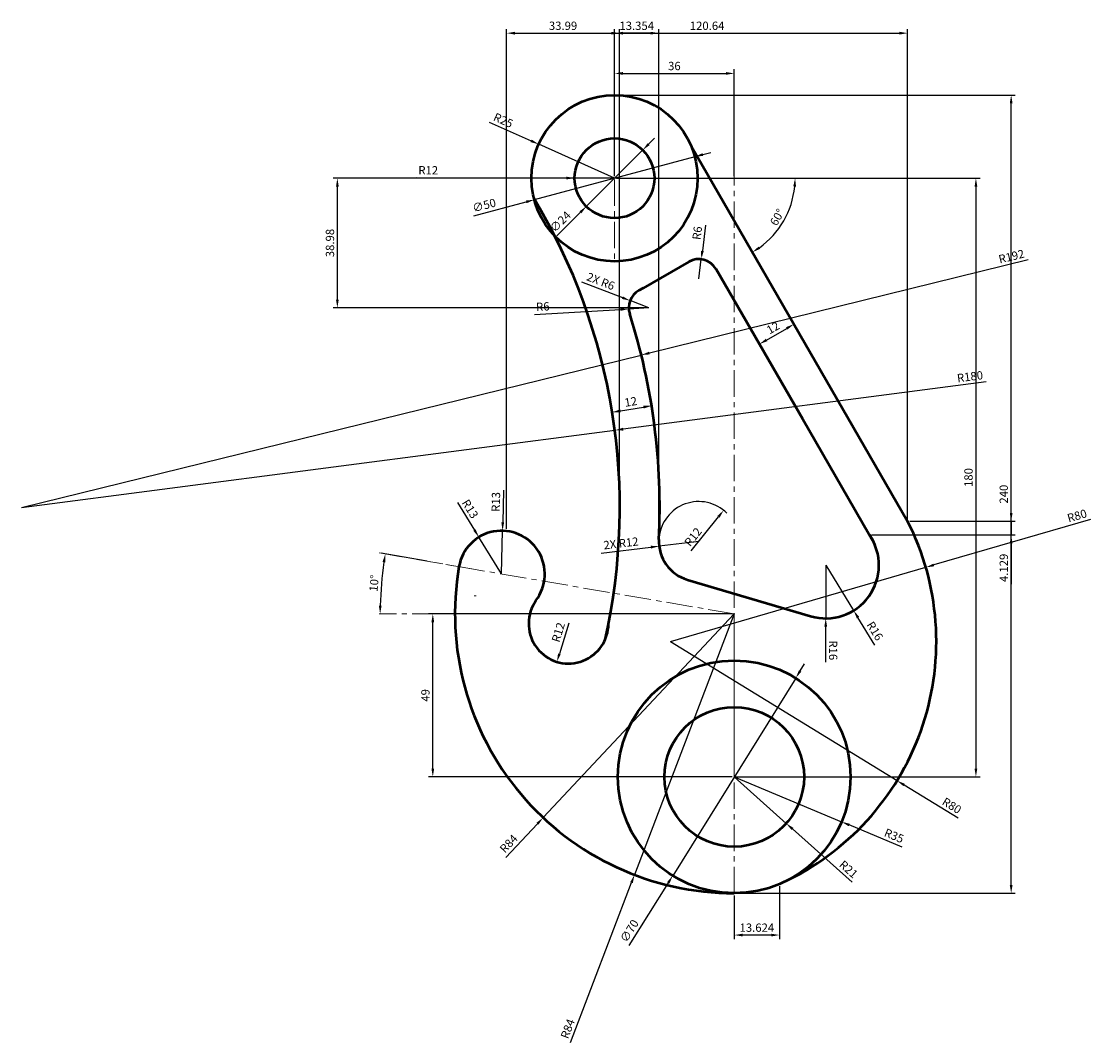
# Model space of a CAD drawing. Units: millimetres. Extents: x 2715 to 3037, y 1203 to 1510.
import ezdxf

# ---------------------------------------------------------------- set-up
doc = ezdxf.new("R2010")
doc.units = ezdxf.units.MM
doc.linetypes.add('CENTER', pattern=[50.8, 31.75, -6.35, 6.35, -6.35])
for name, color, linetype, lineweight in [('M-CNTR', 4, 'CENTER', 18), ('M-CONS', 8, 'Continuous', 13), ('M-DIMS', 2, 'Continuous', 25), ('M-OUTL', 7, 'Continuous', 50)]:
    doc.layers.add(name, color=color, linetype=linetype, lineweight=lineweight)
doc.styles.get("Standard").update_dxf_attribs({"font": 'arial.ttf'})
doc.dimstyles.new('ISO-25', dxfattribs={"dimtxt": 2.5, "dimasz": 2.5, "dimexe": 1.25, "dimexo": 0.625, "dimtad": 1, "dimtxsty": 'Standard', "dimcen": 2.5, "dimadec": 0, "dimazin": 0, "dimtfac": 1, "dimtmove": 0, "dimatfit": 3, "dimfxl": 1, "dimarcsym": 0})

# ---------------------------------------------------------------- blocks, each defined once
blk = doc.blocks.new('*D1')
at = {"layer": 'Defpoints', "color": 0, "transparency": 16777216}
for p in [(2929.68, 1494.7), (2893.68, 1463.19), (2929.68, 1463.19)]:
    blk.add_point(p, dxfattribs=at)
at = {"layer": 'M-DIMS', "color": 0, "lineweight": -2, "transparency": 16777216}
for p, q in [((2893.68, 1463.82), (2893.68, 1495.95)), ((2929.68, 1463.82), (2929.68, 1495.95)), ((2896.18, 1494.7), (2927.18, 1494.7))]:
    blk.add_line(p, q, dxfattribs=at)
at = {"layer": 'M-DIMS', "color": 0, "transparency": 16777216}
for points in [[(2896.18, 1495.12), (2896.18, 1494.29), (2893.68, 1494.7)], [(2927.18, 1495.12), (2927.18, 1494.29), (2929.68, 1494.7)]]:
    blk.add_solid(points, dxfattribs=at)
at = {"layer": 'M-DIMS', "color": 0, "transparency": 16777216, "insert": (2911.68, 1496.61), "char_height": 2.5, "attachment_point": 5}
blk.add_mtext('36', dxfattribs=at)
blk = doc.blocks.new('*D2')
at = {"layer": 'Defpoints', "color": 0, "transparency": 16777216}
for p in [(2947.63, 1419.3), (2947.63, 1419.3), (2937.24, 1413.3)]:
    blk.add_point(p, dxfattribs=at)
at = {"layer": 'M-DIMS', "color": 0, "lineweight": -2, "transparency": 16777216}
for p, q in [((2947.32, 1419.85), (2947.01, 1420.39)), ((2939.41, 1414.55), (2945.47, 1418.05)), ((2936.93, 1413.85), (2936.62, 1414.39))]:
    blk.add_line(p, q, dxfattribs=at)
at = {"layer": 'M-DIMS', "color": 0, "transparency": 16777216}
for points in [[(2945.26, 1418.42), (2945.68, 1417.69), (2947.63, 1419.3)], [(2939.2, 1414.92), (2939.61, 1414.19), (2937.24, 1413.3)]]:
    blk.add_solid(points, dxfattribs=at)
at = {"layer": 'M-DIMS', "color": 0, "transparency": 16777216, "insert": (2941.5, 1417.93), "char_height": 2.5, "attachment_point": 5, "rotation": 30}
blk.add_mtext('12', dxfattribs=at)
blk = doc.blocks.new('*D3')
at = {"layer": 'Defpoints', "color": 0, "transparency": 16777216}
for p in [(2892.98, 1392.85), (2904.83, 1394.76), (2904.83, 1394.76)]:
    blk.add_point(p, dxfattribs=at)
at = {"layer": 'M-DIMS', "color": 0, "lineweight": -2, "transparency": 16777216}
for p, q in [((2904.73, 1395.38), (2904.63, 1395.99)), ((2892.88, 1393.47), (2892.78, 1394.08)), ((2895.45, 1393.25), (2902.36, 1394.36))]:
    blk.add_line(p, q, dxfattribs=at)
at = {"layer": 'M-DIMS', "color": 0, "transparency": 16777216}
for points in [[(2895.38, 1393.66), (2895.52, 1392.84), (2892.98, 1392.85)], [(2902.29, 1394.77), (2902.43, 1393.95), (2904.83, 1394.76)]]:
    blk.add_solid(points, dxfattribs=at)
at = {"layer": 'M-DIMS', "color": 0, "transparency": 16777216, "insert": (2898.61, 1395.66), "char_height": 2.5, "attachment_point": 5, "rotation": 9.1552}
blk.add_mtext('12', dxfattribs=at)
blk = doc.blocks.new('*D4')
at = {"layer": 'Defpoints', "color": 0, "transparency": 16777216}
for p in [(2839.02, 1332.19), (2929.68, 1332.19), (2929.68, 1283.19)]:
    blk.add_point(p, dxfattribs=at)
at = {"layer": 'M-DIMS', "color": 0, "lineweight": -2, "transparency": 16777216}
for p, q in [((2929.05, 1332.19), (2837.77, 1332.19)), ((2839.02, 1285.69), (2839.02, 1329.69)), ((2929.05, 1283.19), (2837.77, 1283.19))]:
    blk.add_line(p, q, dxfattribs=at)
at = {"layer": 'M-DIMS', "color": 0, "transparency": 16777216}
for points in [[(2838.6, 1329.69), (2839.43, 1329.69), (2839.02, 1332.19)], [(2838.6, 1285.69), (2839.43, 1285.69), (2839.02, 1283.19)]]:
    blk.add_solid(points, dxfattribs=at)
at = {"layer": 'M-DIMS', "color": 0, "transparency": 16777216, "insert": (2837.12, 1307.69), "char_height": 2.5, "attachment_point": 5, "rotation": 90}
blk.add_mtext('49', dxfattribs=at)
blk = doc.blocks.new('*D5')
at = {"layer": 'Defpoints', "color": 0, "transparency": 16777216}
for p in [(2870.86, 1473.41), (2893.68, 1463.19)]:
    blk.add_point(p, dxfattribs=at)
at = {"layer": 'M-DIMS', "color": 0, "lineweight": -2, "transparency": 16777216}
for p, q in [((2856, 1480.06), (2868.58, 1474.43)), ((2893.68, 1463.19), (2870.86, 1473.41))]:
    blk.add_line(p, q, dxfattribs=at)
at = {"layer": 'M-DIMS', "color": 0, "transparency": 16777216}
blk.add_solid([(2868.75, 1474.81), (2868.41, 1474.05), (2870.86, 1473.41)], dxfattribs=at)
at = {"layer": 'M-DIMS', "color": 0, "transparency": 16777216, "insert": (2860.08, 1480.31), "char_height": 2.5, "attachment_point": 5, "rotation": 335.8841}
blk.add_mtext('R25', dxfattribs=at)
blk = doc.blocks.new('*D6')
at = {"layer": 'Defpoints', "color": 0, "transparency": 16777216}
for p in [(2881.68, 1463.23), (2893.68, 1463.19)]:
    blk.add_point(p, dxfattribs=at)
at = {"layer": 'M-DIMS', "color": 0, "lineweight": -2, "transparency": 16777216}
for p, q in [((2834.03, 1463.39), (2879.18, 1463.24)), ((2893.68, 1463.19), (2881.68, 1463.23))]:
    blk.add_line(p, q, dxfattribs=at)
at = {"layer": 'M-DIMS', "color": 0, "transparency": 16777216}
blk.add_solid([(2879.18, 1463.66), (2879.18, 1462.82), (2881.68, 1463.23)], dxfattribs=at)
at = {"layer": 'M-DIMS', "color": 0, "transparency": 16777216, "insert": (2837.64, 1465.26), "char_height": 2.5, "attachment_point": 5, "rotation": 359.812}
blk.add_mtext('R12', dxfattribs=at)
blk = doc.blocks.new('*D7')
at = {"layer": 'Defpoints', "color": 0, "transparency": 16777216}
for p in [(2897.97, 1423.87), (2903.96, 1424.21)]:
    blk.add_point(p, dxfattribs=at)
at = {"layer": 'M-DIMS', "color": 0, "lineweight": -2, "transparency": 16777216}
for p, q in [((2869.58, 1422.22), (2895.48, 1423.72)), ((2903.96, 1424.21), (2897.97, 1423.87))]:
    blk.add_line(p, q, dxfattribs=at)
at = {"layer": 'M-DIMS', "color": 0, "transparency": 16777216}
blk.add_solid([(2895.45, 1424.14), (2895.5, 1423.31), (2897.97, 1423.87)], dxfattribs=at)
at = {"layer": 'M-DIMS', "color": 0, "transparency": 16777216, "insert": (2872.11, 1424.27), "char_height": 2.5, "attachment_point": 5, "rotation": 3.3127}
blk.add_mtext('R6', dxfattribs=at)
blk = doc.blocks.new('*D8')
at = {"layer": 'Defpoints', "color": 0, "transparency": 16777216}
for p in [(2919.77, 1438.85), (2919, 1432.9)]:
    blk.add_point(p, dxfattribs=at)
at = {"layer": 'M-DIMS', "color": 0, "lineweight": -2, "transparency": 16777216}
for p, q in [((2921.08, 1449.04), (2920.09, 1441.33)), ((2919, 1432.9), (2919.77, 1438.85))]:
    blk.add_line(p, q, dxfattribs=at)
at = {"layer": 'M-DIMS', "color": 0, "transparency": 16777216}
blk.add_solid([(2919.68, 1441.38), (2920.5, 1441.27), (2919.77, 1438.85)], dxfattribs=at)
at = {"layer": 'M-DIMS', "color": 0, "transparency": 16777216, "insert": (2918.86, 1446.67), "char_height": 2.5, "attachment_point": 5, "rotation": 82.6587}
blk.add_mtext('R6', dxfattribs=at)
blk = doc.blocks.new('*D9')
at = {"layer": 'Defpoints', "color": 0, "transparency": 16777216}
for p in [(2957.19, 1346.85), (2965.58, 1333.23)]:
    blk.add_point(p, dxfattribs=at)
at = {"layer": 'M-DIMS', "color": 0, "lineweight": -2, "transparency": 16777216}
for p, q in [((2957.19, 1346.85), (2965.58, 1333.23)), ((2971.99, 1322.82), (2966.89, 1331.1))]:
    blk.add_line(p, q, dxfattribs=at)
at = {"layer": 'M-DIMS', "color": 0, "transparency": 16777216}
blk.add_solid([(2967.25, 1331.32), (2966.54, 1330.88), (2965.58, 1333.23)], dxfattribs=at)
at = {"layer": 'M-DIMS', "color": 0, "transparency": 16777216, "insert": (2971.71, 1326.89), "char_height": 2.5, "attachment_point": 5, "rotation": 301.6242}
blk.add_mtext('R16', dxfattribs=at)
blk = doc.blocks.new('*D10')
at = {"layer": 'Defpoints', "color": 0, "transparency": 16777216}
for p in [(2926.5, 1363.35), (2919.02, 1353.97)]:
    blk.add_point(p, dxfattribs=at)
at = {"layer": 'M-DIMS', "color": 0, "lineweight": -2, "transparency": 16777216}
blk.add_line((2916.77, 1351.15), (2924.94, 1361.39), dxfattribs=at)
blk.add_arc((2919.02, 1353.97), 12, 45.4603, 174.137, dxfattribs=at)
at = {"layer": 'M-DIMS', "color": 0, "transparency": 16777216}
blk.add_solid([(2924.61, 1361.65), (2925.27, 1361.13), (2926.5, 1363.35)], dxfattribs=at)
at = {"layer": 'M-DIMS', "color": 0, "transparency": 16777216, "insert": (2917.55, 1355.14), "char_height": 2.5, "attachment_point": 5, "rotation": 51.4286}
blk.add_mtext('R12', dxfattribs=at)
blk = doc.blocks.new('*D11')
at = {"layer": 'Defpoints', "color": 0, "transparency": 16777216}
for p in [(2879.85, 1329.27), (2876.36, 1317.78)]:
    blk.add_point(p, dxfattribs=at)
at = {"layer": 'M-DIMS', "color": 0, "lineweight": -2, "transparency": 16777216}
blk.add_line((2879.91, 1329.45), (2877.09, 1320.17), dxfattribs=at)
at = {"layer": 'M-DIMS', "color": 0, "transparency": 16777216}
blk.add_solid([(2876.69, 1320.3), (2877.49, 1320.05), (2876.36, 1317.78)], dxfattribs=at)
at = {"layer": 'M-DIMS', "color": 0, "transparency": 16777216, "insert": (2877.06, 1326.56), "char_height": 2.5, "attachment_point": 5, "rotation": 73.109}
blk.add_mtext('R12', dxfattribs=at)
blk = doc.blocks.new('*D12')
at = {"layer": 'Defpoints', "color": 0, "transparency": 16777216}
for p in [(2852.87, 1355.26), (2859.7, 1344.2)]:
    blk.add_point(p, dxfattribs=at)
at = {"layer": 'M-DIMS', "color": 0, "lineweight": -2, "transparency": 16777216}
for p, q in [((2846.46, 1365.67), (2851.56, 1357.39)), ((2859.7, 1344.2), (2852.87, 1355.26))]:
    blk.add_line(p, q, dxfattribs=at)
at = {"layer": 'M-DIMS', "color": 0, "transparency": 16777216}
blk.add_solid([(2851.92, 1357.61), (2851.21, 1357.17), (2852.87, 1355.26)], dxfattribs=at)
at = {"layer": 'M-DIMS', "color": 0, "transparency": 16777216, "insert": (2849.97, 1363.59), "char_height": 2.5, "attachment_point": 5, "rotation": 301.6763}
blk.add_mtext('R13', dxfattribs=at)
blk = doc.blocks.new('*D13')
at = {"layer": 'Defpoints', "color": 0, "transparency": 16777216}
for p in [(2929.68, 1332.19), (2872.21, 1270.93)]:
    blk.add_point(p, dxfattribs=at)
at = {"layer": 'M-DIMS', "color": 0, "lineweight": -2, "transparency": 16777216}
for p, q in [((2929.68, 1332.19), (2872.21, 1270.93)), ((2860.99, 1258.97), (2870.5, 1269.1))]:
    blk.add_line(p, q, dxfattribs=at)
at = {"layer": 'M-DIMS', "color": 0, "transparency": 16777216}
blk.add_solid([(2870.2, 1269.39), (2870.8, 1268.82), (2872.21, 1270.93)], dxfattribs=at)
at = {"layer": 'M-DIMS', "color": 0, "transparency": 16777216, "insert": (2862.07, 1262.9), "char_height": 2.5, "attachment_point": 5, "rotation": 46.8317}
blk.add_mtext('R84', dxfattribs=at)
blk = doc.blocks.new('*D14')
at = {"layer": 'Defpoints', "color": 0, "transparency": 16777216}
for p in [(2929.68, 1283.19), (2945.33, 1269.2)]:
    blk.add_point(p, dxfattribs=at)
at = {"layer": 'M-DIMS', "color": 0, "lineweight": -2, "transparency": 16777216}
for p, q in [((2929.68, 1283.19), (2945.33, 1269.2)), ((2965.11, 1251.52), (2947.2, 1267.53))]:
    blk.add_line(p, q, dxfattribs=at)
at = {"layer": 'M-DIMS', "color": 0, "transparency": 16777216}
blk.add_solid([(2947.48, 1267.84), (2946.92, 1267.22), (2945.33, 1269.2)], dxfattribs=at)
at = {"layer": 'M-DIMS', "color": 0, "transparency": 16777216, "insert": (2963.85, 1255.17), "char_height": 2.5, "attachment_point": 5, "rotation": 318.2044}
blk.add_mtext('R21', dxfattribs=at)
blk = doc.blocks.new('*D15')
at = {"layer": 'Defpoints', "color": 0, "transparency": 16777216}
for p in [(2929.68, 1283.19), (2961.97, 1269.68)]:
    blk.add_point(p, dxfattribs=at)
at = {"layer": 'M-DIMS', "color": 0, "lineweight": -2, "transparency": 16777216}
for p, q in [((2929.68, 1283.19), (2961.97, 1269.68)), ((2980.23, 1262.04), (2964.27, 1268.72))]:
    blk.add_line(p, q, dxfattribs=at)
at = {"layer": 'M-DIMS', "color": 0, "transparency": 16777216}
blk.add_solid([(2964.43, 1269.1), (2964.11, 1268.33), (2961.97, 1269.68)], dxfattribs=at)
at = {"layer": 'M-DIMS', "color": 0, "transparency": 16777216, "insert": (2977.63, 1265.19), "char_height": 2.5, "attachment_point": 5, "rotation": 337.2957}
blk.add_mtext('R35', dxfattribs=at)
blk = doc.blocks.new('*D16')
at = {"layer": 'Defpoints', "color": 0, "transparency": 16777216}
for p in [(2910.47, 1323.91), (2978.64, 1282.05)]:
    blk.add_point(p, dxfattribs=at)
at = {"layer": 'M-DIMS', "color": 0, "lineweight": -2, "transparency": 16777216}
for p, q in [((2910.47, 1323.91), (2978.64, 1282.05)), ((2997.03, 1270.76), (2980.77, 1280.74))]:
    blk.add_line(p, q, dxfattribs=at)
at = {"layer": 'M-DIMS', "color": 0, "transparency": 16777216}
blk.add_solid([(2980.99, 1281.1), (2980.56, 1280.39), (2978.64, 1282.05)], dxfattribs=at)
at = {"layer": 'M-DIMS', "color": 0, "transparency": 16777216, "insert": (2994.95, 1274.27), "char_height": 2.5, "attachment_point": 5, "rotation": 328.4483}
blk.add_mtext('R80', dxfattribs=at)
blk = doc.blocks.new('*D17')
at = {"layer": 'Defpoints', "color": 0, "transparency": 16777216}
for p in [(2916.78, 1472.74), (2929.68, 1463.19), (2984.65, 1463.19), (2941.97, 1446.68), (2960.68, 1396.71)]:
    blk.add_point(p, dxfattribs=at)
at = {"layer": 'M-DIMS', "color": 0, "lineweight": -2, "transparency": 16777216}
blk.add_arc((2922.3, 1463.19), 25.69, 305.5787, 354.4213, dxfattribs=at)
at = {"layer": 'M-DIMS', "color": 0, "transparency": 16777216}
for points in [[(2947.44, 1460.72), (2948.28, 1460.68), (2947.98, 1463.19)], [(2937.47, 1441.95), (2937.01, 1442.65), (2935.14, 1440.95)]]:
    blk.add_solid(points, dxfattribs=at)
at = {"layer": 'M-DIMS', "color": 0, "transparency": 16777216, "insert": (2942.89, 1451.3), "char_height": 2.5, "attachment_point": 5, "rotation": 60}
blk.add_mtext('60°', dxfattribs=at)
blk = doc.blocks.new('*D18')
at = {"layer": 'Defpoints', "color": 0, "transparency": 16777216}
for p in [(2837.98, 1347.93), (2850.79, 1345.73), (2823.86, 1344.23), (2822.88, 1332.19), (2929.68, 1332.19)]:
    blk.add_point(p, dxfattribs=at)
at = {"layer": 'M-DIMS', "color": 0, "lineweight": -2, "transparency": 16777216}
blk.add_line((2837.36, 1348.03), (2823.48, 1350.41), dxfattribs=at)
blk.add_arc((2929.82, 1332.19), 106.64, 171.6214, 178.6568, dxfattribs=at)
at = {"layer": 'M-DIMS', "color": 0, "transparency": 16777216}
for points in [[(2823.9, 1347.8), (2824.73, 1347.67), (2824.71, 1350.2)], [(2823.62, 1334.69), (2822.79, 1334.7), (2823.18, 1332.19)]]:
    blk.add_solid(points, dxfattribs=at)
at = {"layer": 'M-DIMS', "color": 0, "transparency": 16777216, "insert": (2821.67, 1341.39), "char_height": 2.5, "attachment_point": 5, "rotation": 85.1391}
blk.add_mtext('10°', dxfattribs=at)
blk = doc.blocks.new('*D19')
at = {"layer": 'Defpoints', "color": 0, "transparency": 16777216}
for p in [(2893.68, 1463.19), (2929.68, 1283.19), (3002.37, 1283.19)]:
    blk.add_point(p, dxfattribs=at)
at = {"layer": 'M-DIMS', "color": 0, "lineweight": -2, "transparency": 16777216}
for p, q in [((2894.3, 1463.19), (3003.62, 1463.19)), ((3002.37, 1460.69), (3002.37, 1285.69)), ((2930.3, 1283.19), (3003.62, 1283.19))]:
    blk.add_line(p, q, dxfattribs=at)
at = {"layer": 'M-DIMS', "color": 0, "transparency": 16777216}
for points in [[(3001.96, 1460.69), (3002.79, 1460.69), (3002.37, 1463.19)], [(3001.96, 1285.69), (3002.79, 1285.69), (3002.37, 1283.19)]]:
    blk.add_solid(points, dxfattribs=at)
at = {"layer": 'M-DIMS', "color": 0, "transparency": 16777216, "insert": (3000.47, 1373.19), "char_height": 2.5, "attachment_point": 5, "rotation": 90}
blk.add_mtext('180', dxfattribs=at)
blk = doc.blocks.new('*D20')
at = {"layer": 'Defpoints', "color": 0, "transparency": 16777216}
for p in [(2893.68, 1488.19), (3012.97, 1488.19), (2929.68, 1248.19)]:
    blk.add_point(p, dxfattribs=at)
at = {"layer": 'M-DIMS', "color": 0, "lineweight": -2, "transparency": 16777216}
for p, q in [((2894.3, 1488.19), (3014.22, 1488.19)), ((3012.97, 1250.69), (3012.97, 1485.69)), ((2930.3, 1248.19), (3014.22, 1248.19))]:
    blk.add_line(p, q, dxfattribs=at)
at = {"layer": 'M-DIMS', "color": 0, "transparency": 16777216}
for points in [[(3012.56, 1485.69), (3013.39, 1485.69), (3012.97, 1488.19)], [(3012.56, 1250.69), (3013.39, 1250.69), (3012.97, 1248.19)]]:
    blk.add_solid(points, dxfattribs=at)
at = {"layer": 'M-DIMS', "color": 0, "transparency": 16777216, "insert": (3011.07, 1368.19), "char_height": 2.5, "attachment_point": 5, "rotation": 90}
blk.add_mtext('240', dxfattribs=at)
blk = doc.blocks.new('*D21')
at = {"layer": 'Defpoints', "color": 0, "transparency": 16777216}
for p in [(2929.68, 1248.19), (2943.3, 1250.94), (2929.68, 1235.63)]:
    blk.add_point(p, dxfattribs=at)
at = {"layer": 'M-DIMS', "color": 0, "lineweight": -2, "transparency": 16777216}
for p, q in [((2943.3, 1250.32), (2943.3, 1234.38)), ((2929.68, 1247.57), (2929.68, 1234.38)), ((2940.8, 1235.63), (2932.18, 1235.63))]:
    blk.add_line(p, q, dxfattribs=at)
at = {"layer": 'M-DIMS', "color": 0, "transparency": 16777216}
for points in [[(2932.18, 1236.04), (2932.18, 1235.21), (2929.68, 1235.63)], [(2940.8, 1236.04), (2940.8, 1235.21), (2943.3, 1235.63)]]:
    blk.add_solid(points, dxfattribs=at)
at = {"layer": 'M-DIMS', "color": 0, "transparency": 16777216, "insert": (2936.49, 1237.53), "char_height": 2.5, "attachment_point": 5}
blk.add_mtext('13.624', dxfattribs=at)
blk = doc.blocks.new('*D22')
at = {"layer": 'Defpoints', "color": 0, "transparency": 16777216}
for p in [(2981.84, 1360.05), (2970.37, 1355.93), (3012.97, 1355.93)]:
    blk.add_point(p, dxfattribs=at)
at = {"layer": 'M-DIMS', "color": 0, "lineweight": -2, "transparency": 16777216}
for p, q in [((3012.97, 1362.55), (3012.97, 1365.05)), ((2982.47, 1360.05), (3014.22, 1360.05)), ((3012.97, 1360.05), (3012.97, 1355.93)), ((2970.99, 1355.93), (3014.22, 1355.93)), ((3012.97, 1353.43), (3012.97, 1341.13))]:
    blk.add_line(p, q, dxfattribs=at)
at = {"layer": 'M-DIMS', "color": 0, "transparency": 16777216}
for points in [[(3012.56, 1362.55), (3013.39, 1362.55), (3012.97, 1360.05)], [(3012.56, 1353.43), (3013.39, 1353.43), (3012.97, 1355.93)]]:
    blk.add_solid(points, dxfattribs=at)
at = {"layer": 'M-DIMS', "color": 0, "transparency": 16777216, "insert": (3011.07, 1346.03), "char_height": 2.5, "attachment_point": 5, "rotation": 90}
blk.add_mtext('4.129', dxfattribs=at)
blk = doc.blocks.new('*D23')
at = {"layer": 'Defpoints', "color": 0, "transparency": 16777216}
for p in [(2893.68, 1506.81), (2893.68, 1488.19), (2907.03, 1354.57)]:
    blk.add_point(p, dxfattribs=at)
at = {"layer": 'M-DIMS', "color": 0, "lineweight": -2, "transparency": 16777216}
for p, q in [((2893.68, 1488.82), (2893.68, 1508.06)), ((2904.53, 1506.81), (2896.18, 1506.81)), ((2907.03, 1355.19), (2907.03, 1508.06))]:
    blk.add_line(p, q, dxfattribs=at)
at = {"layer": 'M-DIMS', "color": 0, "transparency": 16777216}
for points in [[(2896.18, 1507.22), (2896.18, 1506.39), (2893.68, 1506.81)], [(2904.53, 1507.22), (2904.53, 1506.39), (2907.03, 1506.81)]]:
    blk.add_solid(points, dxfattribs=at)
at = {"layer": 'M-DIMS', "color": 0, "transparency": 16777216, "insert": (2900.35, 1508.71), "char_height": 2.5, "attachment_point": 5}
blk.add_mtext('13.354', dxfattribs=at)
blk = doc.blocks.new('*D24')
at = {"layer": 'Defpoints', "color": 0, "transparency": 16777216}
for p in [(2895.19, 1506.81), (2895.19, 1358.67), (2861.2, 1357.11)]:
    blk.add_point(p, dxfattribs=at)
at = {"layer": 'M-DIMS', "color": 0, "lineweight": -2, "transparency": 16777216}
for p, q in [((2861.2, 1357.74), (2861.2, 1508.06)), ((2863.7, 1506.81), (2892.69, 1506.81)), ((2895.19, 1359.3), (2895.19, 1508.06))]:
    blk.add_line(p, q, dxfattribs=at)
at = {"layer": 'M-DIMS', "color": 0, "transparency": 16777216}
for points in [[(2863.7, 1507.22), (2863.7, 1506.39), (2861.2, 1506.81)], [(2892.69, 1507.22), (2892.69, 1506.39), (2895.19, 1506.81)]]:
    blk.add_solid(points, dxfattribs=at)
at = {"layer": 'M-DIMS', "color": 0, "transparency": 16777216, "insert": (2878.19, 1508.71), "char_height": 2.5, "attachment_point": 5}
blk.add_mtext('33.99', dxfattribs=at)
blk = doc.blocks.new('*D25')
at = {"layer": 'Defpoints', "color": 0, "transparency": 16777216}
for p in [(2810.31, 1463.19), (2893.68, 1463.19), (2903.96, 1424.21)]:
    blk.add_point(p, dxfattribs=at)
at = {"layer": 'M-DIMS', "color": 0, "lineweight": -2, "transparency": 16777216}
for p, q in [((2893.05, 1463.19), (2809.06, 1463.19)), ((2810.31, 1426.71), (2810.31, 1460.69)), ((2903.34, 1424.21), (2809.06, 1424.21))]:
    blk.add_line(p, q, dxfattribs=at)
at = {"layer": 'M-DIMS', "color": 0, "transparency": 16777216}
for points in [[(2809.9, 1460.69), (2810.73, 1460.69), (2810.31, 1463.19)], [(2809.9, 1426.71), (2810.73, 1426.71), (2810.31, 1424.21)]]:
    blk.add_solid(points, dxfattribs=at)
at = {"layer": 'M-DIMS', "color": 0, "transparency": 16777216, "insert": (2808.41, 1443.7), "char_height": 2.5, "attachment_point": 5, "rotation": 90}
blk.add_mtext('38.98', dxfattribs=at)
blk = doc.blocks.new('*D26')
at = {"layer": 'Defpoints', "color": 0, "transparency": 16777216}
for p in [(2981.84, 1506.81), (2981.84, 1360.05), (2861.2, 1357.11)]:
    blk.add_point(p, dxfattribs=at)
at = {"layer": 'M-DIMS', "color": 0, "lineweight": -2, "transparency": 16777216}
for p, q in [((2861.2, 1357.74), (2861.2, 1508.06)), ((2863.7, 1506.81), (2979.34, 1506.81)), ((2981.84, 1360.68), (2981.84, 1508.06))]:
    blk.add_line(p, q, dxfattribs=at)
at = {"layer": 'M-DIMS', "color": 0, "transparency": 16777216}
for points in [[(2863.7, 1507.22), (2863.7, 1506.39), (2861.2, 1506.81)], [(2979.34, 1507.22), (2979.34, 1506.39), (2981.84, 1506.81)]]:
    blk.add_solid(points, dxfattribs=at)
at = {"layer": 'M-DIMS', "color": 0, "transparency": 16777216, "insert": (2921.52, 1508.71), "char_height": 2.5, "attachment_point": 5}
blk.add_mtext('120.64', dxfattribs=at)
blk = doc.blocks.new('*D27')
at = {"layer": 'Defpoints', "color": 0, "transparency": 16777216}
for p in [(2917.83, 1469.67), (2869.53, 1456.72)]:
    blk.add_point(p, dxfattribs=at)
at = {"layer": 'M-DIMS', "color": 0, "lineweight": -2, "transparency": 16777216}
for p, q in [((2920.24, 1470.31), (2922.66, 1470.96)), ((2917.83, 1469.67), (2869.53, 1456.72)), ((2851.4, 1451.86), (2867.12, 1456.07))]:
    blk.add_line(p, q, dxfattribs=at)
at = {"layer": 'M-DIMS', "color": 0, "transparency": 16777216}
for points in [[(2920.13, 1470.71), (2920.35, 1469.91), (2917.83, 1469.67)], [(2867.01, 1456.48), (2867.22, 1455.67), (2869.53, 1456.72)]]:
    blk.add_solid(points, dxfattribs=at)
at = {"layer": 'M-DIMS', "color": 0, "transparency": 16777216, "insert": (2854.53, 1454.74), "char_height": 2.5, "attachment_point": 5, "rotation": 15.005}
blk.add_mtext('∅50', dxfattribs=at)
blk = doc.blocks.new('*D28')
at = {"layer": 'Defpoints', "color": 0, "transparency": 16777216}
for p in [(2902.17, 1471.68), (2885.19, 1454.71)]:
    blk.add_point(p, dxfattribs=at)
at = {"layer": 'M-DIMS', "color": 0, "lineweight": -2, "transparency": 16777216}
for p, q in [((2903.93, 1473.44), (2905.7, 1475.21)), ((2902.17, 1471.68), (2885.19, 1454.71)), ((2876.32, 1445.85), (2883.42, 1452.94))]:
    blk.add_line(p, q, dxfattribs=at)
at = {"layer": 'M-DIMS', "color": 0, "transparency": 16777216}
for points in [[(2903.64, 1473.74), (2904.23, 1473.15), (2902.17, 1471.68)], [(2883.13, 1453.24), (2883.72, 1452.65), (2885.19, 1454.71)]]:
    blk.add_solid(points, dxfattribs=at)
at = {"layer": 'M-DIMS', "color": 0, "transparency": 16777216, "insert": (2877.59, 1449.9), "char_height": 2.5, "attachment_point": 5, "rotation": 44.9821}
blk.add_mtext('∅24', dxfattribs=at)
blk = doc.blocks.new('*D29')
at = {"layer": 'Defpoints', "color": 0, "transparency": 16777216}
for p in [(2948.18, 1312.9), (2911.18, 1253.48)]:
    blk.add_point(p, dxfattribs=at)
at = {"layer": 'M-DIMS', "color": 0, "lineweight": -2, "transparency": 16777216}
for p, q in [((2949.5, 1315.03), (2950.82, 1317.15)), ((2948.18, 1312.9), (2911.18, 1253.48)), ((2898.09, 1232.45), (2909.86, 1251.36))]:
    blk.add_line(p, q, dxfattribs=at)
at = {"layer": 'M-DIMS', "color": 0, "transparency": 16777216}
for points in [[(2949.14, 1315.25), (2949.85, 1314.81), (2948.18, 1312.9)], [(2909.5, 1251.58), (2910.21, 1251.14), (2911.18, 1253.48)]]:
    blk.add_solid(points, dxfattribs=at)
at = {"layer": 'M-DIMS', "color": 0, "transparency": 16777216, "insert": (2898.41, 1236.7), "char_height": 2.5, "attachment_point": 5, "rotation": 58.0924}
blk.add_mtext('∅70', dxfattribs=at)
blk = doc.blocks.new('*D30')
at = {"layer": 'Defpoints', "color": 0, "transparency": 16777216}
for p in [(2929.68, 1332.19), (2899.68, 1253.73)]:
    blk.add_point(p, dxfattribs=at)
at = {"layer": 'M-DIMS', "color": 0, "lineweight": -2, "transparency": 16777216}
for p, q in [((2929.68, 1332.19), (2899.68, 1253.73)), ((2880.39, 1203.29), (2898.78, 1251.4))]:
    blk.add_line(p, q, dxfattribs=at)
at = {"layer": 'M-DIMS', "color": 0, "transparency": 16777216}
blk.add_solid([(2898.4, 1251.55), (2899.17, 1251.25), (2899.68, 1253.73)], dxfattribs=at)
at = {"layer": 'M-DIMS', "color": 0, "transparency": 16777216, "insert": (2879.9, 1207.34), "char_height": 2.5, "attachment_point": 5, "rotation": 69.0748}
blk.add_mtext('R84', dxfattribs=at)
blk = doc.blocks.new('*D31')
at = {"layer": 'Defpoints', "color": 0, "transparency": 16777216}
for p in [(2987.3, 1346.2), (2910.47, 1323.91)]:
    blk.add_point(p, dxfattribs=at)
at = {"layer": 'M-DIMS', "color": 0, "lineweight": -2, "transparency": 16777216}
for p, q in [((3036.87, 1360.58), (2989.7, 1346.9)), ((2910.47, 1323.91), (2987.3, 1346.2))]:
    blk.add_line(p, q, dxfattribs=at)
at = {"layer": 'M-DIMS', "color": 0, "transparency": 16777216}
blk.add_solid([(2989.59, 1347.3), (2989.82, 1346.5), (2987.3, 1346.2)], dxfattribs=at)
at = {"layer": 'M-DIMS', "color": 0, "transparency": 16777216, "insert": (3032.87, 1361.4), "char_height": 2.5, "attachment_point": 5, "rotation": 16.1759}
blk.add_mtext('R80', dxfattribs=at)
blk = doc.blocks.new('*D32')
at = {"layer": 'Defpoints', "color": 0, "transparency": 16777216}
for p in [(2957.19, 1346.85), (2957.2, 1330.85)]:
    blk.add_point(p, dxfattribs=at)
at = {"layer": 'M-DIMS', "color": 0, "lineweight": -2, "transparency": 16777216}
for p, q in [((2957.19, 1346.85), (2957.2, 1330.85)), ((2957.21, 1317.64), (2957.2, 1328.35))]:
    blk.add_line(p, q, dxfattribs=at)
at = {"layer": 'M-DIMS', "color": 0, "transparency": 16777216}
blk.add_solid([(2957.62, 1328.35), (2956.78, 1328.35), (2957.2, 1330.85)], dxfattribs=at)
at = {"layer": 'M-DIMS', "color": 0, "transparency": 16777216, "insert": (2959.11, 1321.25), "char_height": 2.5, "attachment_point": 5, "rotation": 270.0323}
blk.add_mtext('R16', dxfattribs=at)
blk = doc.blocks.new('*D33')
at = {"layer": 'Defpoints', "color": 0, "transparency": 16777216}
for p in [(2860, 1357.2), (2859.7, 1344.2)]:
    blk.add_point(p, dxfattribs=at)
at = {"layer": 'M-DIMS', "color": 0, "lineweight": -2, "transparency": 16777216}
for p, q in [((2860.28, 1369.42), (2860.06, 1359.69)), ((2859.7, 1344.2), (2860, 1357.2))]:
    blk.add_line(p, q, dxfattribs=at)
at = {"layer": 'M-DIMS', "color": 0, "transparency": 16777216}
blk.add_solid([(2859.64, 1359.7), (2860.47, 1359.69), (2860, 1357.2)], dxfattribs=at)
at = {"layer": 'M-DIMS', "color": 0, "transparency": 16777216, "insert": (2858.3, 1365.85), "char_height": 2.5, "attachment_point": 5, "rotation": 88.6793}
blk.add_mtext('R13', dxfattribs=at)
blk = doc.blocks.new('*D34')
at = {"layer": 'Defpoints', "color": 0, "transparency": 16777216}
for p in [(2919.02, 1353.97), (2907.1, 1352.56)]:
    blk.add_point(p, dxfattribs=at)
at = {"layer": 'M-DIMS', "color": 0, "lineweight": -2, "transparency": 16777216}
for p, q in [((2919.02, 1353.97), (2907.1, 1352.56)), ((2889.61, 1350.49), (2904.62, 1352.26))]:
    blk.add_line(p, q, dxfattribs=at)
at = {"layer": 'M-DIMS', "color": 0, "transparency": 16777216}
blk.add_solid([(2904.57, 1352.68), (2904.67, 1351.85), (2907.1, 1352.56)], dxfattribs=at)
at = {"layer": 'M-DIMS', "color": 0, "transparency": 16777216, "insert": (2895.65, 1353.1), "char_height": 2.5, "attachment_point": 5, "rotation": 6.7445}
blk.add_mtext('2X R12', dxfattribs=at)
blk = doc.blocks.new('*D35')
at = {"layer": 'Defpoints', "color": 0, "transparency": 16777216}
for p in [(2898.37, 1426.38), (2903.96, 1424.21)]:
    blk.add_point(p, dxfattribs=at)
at = {"layer": 'M-DIMS', "color": 0, "lineweight": -2, "transparency": 16777216}
for p, q in [((2883.74, 1432.05), (2896.04, 1427.28)), ((2903.96, 1424.21), (2898.37, 1426.38))]:
    blk.add_line(p, q, dxfattribs=at)
at = {"layer": 'M-DIMS', "color": 0, "transparency": 16777216}
blk.add_solid([(2896.19, 1427.67), (2895.89, 1426.9), (2898.37, 1426.38)], dxfattribs=at)
at = {"layer": 'M-DIMS', "color": 0, "transparency": 16777216, "insert": (2889.41, 1431.89), "char_height": 2.5, "attachment_point": 5, "rotation": 338.8182}
blk.add_mtext('2X R6', dxfattribs=at)
blk = doc.blocks.new('*D36')
at = {"layer": 'Defpoints', "color": 0, "transparency": 16777216}
for p in [(2893.77, 1387.41), (2715.27, 1364.21)]:
    blk.add_point(p, dxfattribs=at)
at = {"layer": 'M-DIMS', "color": 0, "lineweight": -2, "transparency": 16777216}
for p, q in [((3005.41, 1401.93), (2896.25, 1387.74)), ((2715.27, 1364.21), (2893.77, 1387.41))]:
    blk.add_line(p, q, dxfattribs=at)
at = {"layer": 'M-DIMS', "color": 0, "transparency": 16777216}
blk.add_solid([(2896.2, 1388.15), (2896.31, 1387.32), (2893.77, 1387.41)], dxfattribs=at)
at = {"layer": 'M-DIMS', "color": 0, "transparency": 16777216, "insert": (3000.63, 1403.22), "char_height": 2.5, "attachment_point": 5, "rotation": 7.4062}
blk.add_mtext('R180', dxfattribs=at)
blk = doc.blocks.new('*D37')
at = {"layer": 'Defpoints', "color": 0, "transparency": 16777216}
for p in [(2901.73, 1410.03), (2715.27, 1364.21)]:
    blk.add_point(p, dxfattribs=at)
at = {"layer": 'M-DIMS', "color": 0, "lineweight": -2, "transparency": 16777216}
for p, q in [((3018.04, 1438.61), (2904.15, 1410.63)), ((2715.27, 1364.21), (2901.73, 1410.03))]:
    blk.add_line(p, q, dxfattribs=at)
at = {"layer": 'M-DIMS', "color": 0, "transparency": 16777216}
blk.add_solid([(2904.06, 1411.03), (2904.25, 1410.22), (2901.73, 1410.03)], dxfattribs=at)
at = {"layer": 'M-DIMS', "color": 0, "transparency": 16777216, "insert": (3013.14, 1439.37), "char_height": 2.5, "attachment_point": 5, "rotation": 13.8067}
blk.add_mtext('R192', dxfattribs=at)

msp = doc.modelspace()

# ---------------------------------------------------------------- linework, layer by layer
at = {"layer": 'M-CNTR', "ltscale": 0.25}
for p, q in [((2893.678, 1488.1927), (2893.678, 1438.1927)), ((2929.678, 1463.1927), (2881.678, 1463.1927)), ((2929.678, 1283.1927), (2929.678, 1463.1927)), ((2929.678, 1463.1927), (2984.652, 1463.1927)), ((2929.678, 1332.1927), (2822.8783, 1350.5229)), ((2850.7923, 1345.732), (2837.979, 1347.9272)), ((2929.678, 1332.1927), (2822.8783, 1332.1927)), ((2894.678, 1283.1927), (3000.4087, 1283.1927)), ((2929.678, 1248.1927), (2929.678, 1283.1927))]:
    msp.add_line(p, q, dxfattribs=at)
at = {"layer": 'M-CNTR'}
msp.add_line((2881.678, 1463.1927), (2875.4457, 1463.1927), dxfattribs=at)
at = {"layer": 'M-CONS'}
for p, q in [((2929.678, 1463.1927), (2929.678, 1494.2425)), ((2874.7683, 1446.3133), (2875.0274, 1446.5446)), ((2851.4847, 1337.5962), (2852.0777, 1337.5962)), ((2874.7923, 1332.1927), (2862.7923, 1332.1927)), ((2929.678, 1283.1927), (2929.678, 1332.1927))]:
    msp.add_line(p, q, dxfattribs=at)
at = {"layer": 'M-OUTL'}
for p, q in [((2916.7833, 1472.7396), (2960.6767, 1396.714)), ((2916.0026, 1438.0917), (2902.2752, 1430.1662)), ((2924.1988, 1435.8956), (2950.2844, 1390.714)), ((2902.2752, 1430.1662), (2900.9639, 1429.4091)), ((2960.6767, 1396.714), (2981.8419, 1360.0548)), ((2950.2844, 1390.714), (2972.071, 1352.9785)), ((2915.6152, 1342.4574), (2952.6555, 1331.5085)), ((2869.1349, 1334.6686), (2869.975, 1336.2345))]:
    msp.add_line(p, q, dxfattribs=at)
for centre, radius in [((2893.678, 1463.1927), 25), ((2893.678, 1463.1927), 12), ((2929.678, 1283.1927), 35), ((2929.678, 1283.1927), 21)]:
    msp.add_circle(centre, radius, dxfattribs=at)
for centre, radius, start, end in [((2715.2743, 1364.2109), 180, 347.218499, 31.091942), ((2919.0026, 1432.8956), 6, 30, 120), ((2903.9639, 1424.2129), 6, 120, 197.640326), ((2715.2743, 1364.2109), 192, 357.121169, 17.640326), ((2859.7005, 1344.1991), 13, 322.217583, 170.244053), ((2910.4707, 1323.914), 80, 296.485633, 26.856655), ((2919.0168, 1353.9652), 12, 177.121169, 253.532583), ((2957.191, 1346.8522), 16, 253.532583, 34.548727), ((2929.678, 1332.1927), 84, 170.261112, 270), ((2879.8495, 1329.2651), 12, 153.237676, 0)]:
    msp.add_arc(centre, radius, start, end, dxfattribs=at)

# ---------------------------------------------------------------- dimensions: what is measured, and where the dimension line sits
at = {"layer": 'M-DIMS'}
for base, p1, p2, override, picture, middle in [((2895.1896, 1506.8075), (2861.2, 1357.113), (2895.1896, 1358.6706), {"dimdec": 2, "dimlfac": 1, "dimrnd": 0, "dimzin": 0, "dimdsep": 46, "dimlunit": 2}, '*D24', (2878.1948, 1508.7098)), ((2981.8419, 1506.8075), (2861.2, 1357.113), (2981.8419, 1360.0548), {"dimdec": 2, "dimlfac": 1, "dimrnd": 0, "dimzin": 0, "dimdsep": 46, "dimlunit": 2}, '*D26', (2921.5209, 1508.7089)), ((2893.678, 1506.8075), (2907.032, 1354.5679), (2893.678, 1488.1927), {"dimdec": 3, "dimlfac": 1, "dimrnd": 0, "dimzin": 0, "dimdsep": 46, "dimlunit": 2}, '*D23', (2900.355, 1508.7098)), ((2929.678, 1494.7032), (2893.678, 1463.1927), (2929.678, 1463.1927), {"dimclrd": 0, "dimclre": 0, "dimclrt": 0}, '*D1', (2911.678, 1496.6055)), ((2929.67796, 1235.62767), (2943.30154, 1250.94314), (2929.67796, 1248.19267), {"dimdec": 3, "dimlfac": 1, "dimrnd": 0, "dimzin": 0, "dimdsep": 46, "dimlunit": 2}, '*D21', (2936.48975, 1237.52995))]:
    dim = msp.add_linear_dim(base=base, p1=p1, p2=p2, dimstyle='ISO-25', override=override, dxfattribs=at)
    dim.commit()
    dim.dimension.update_dxf_attribs({"geometry": picture, "text_midpoint": middle})
for base, p1, p2, override, picture, middle in [((3012.9737, 1488.1927), (2929.678, 1248.1927), (2893.678, 1488.1927), {"dimdec": 0, "dimlfac": 1, "dimrnd": 0, "dimzin": 0, "dimdsep": 46, "dimlunit": 2}, '*D20', (3011.0722, 1368.1927)), ((2810.3133, 1463.1927), (2903.9639, 1424.2129), (2893.678, 1463.1927), {"dimdec": 2, "dimlfac": 1, "dimrnd": 0, "dimzin": 0, "dimdsep": 46, "dimlunit": 2}, '*D25', (2808.411, 1443.7028)), ((3002.372, 1283.1927), (2893.678, 1463.1927), (2929.678, 1283.1927), {"dimclrd": 0, "dimclre": 0, "dimclrt": 0}, '*D19', (3000.4705, 1373.1927)), ((3012.9737, 1355.9259), (2981.8419, 1360.0548), (2970.3693, 1355.9259), {"dimdec": 3, "dimlfac": 1, "dimrnd": 0, "dimzin": 0, "dimdsep": 46, "dimlunit": 2}, '*D22', (3011.0722, 1346.0299)), ((2839.0174, 1332.1927), (2929.678, 1283.1927), (2929.678, 1332.1927), {"dimclrd": 0, "dimclre": 0, "dimclrt": 0}, '*D4', (2837.116, 1307.6927))]:
    dim = msp.add_linear_dim(base=base, p1=p1, p2=p2, angle=90, dimstyle='ISO-25', override=override, dxfattribs=at)
    dim.commit()
    dim.dimension.update_dxf_attribs({"geometry": picture, "text_midpoint": middle})
for center, mpoint, override, picture, middle in [((2893.678, 1463.1927), (2870.8599, 1473.4073), {"dimclrd": 0, "dimclre": 0, "dimclrt": 0}, '*D5', (2859.3066, 1478.5792)), ((2893.678, 1463.1927), (2881.678, 1463.232), {"dimclrd": 0, "dimclre": 0, "dimclrt": 0}, '*D6', (2837.634, 1463.3765)), ((2715.2743, 1364.2109), (2901.7267, 1410.0311), {"dimdec": 0, "dimlfac": 1, "dimrnd": 0, "dimzin": 0, "dimdsep": 46, "dimlunit": 2}, '*D37', (3013.5982, 1437.5233)), ((2903.9639, 1424.2129), (2897.9739, 1423.8662), {"dimclrd": 0, "dimclre": 0, "dimclrt": 0}, '*D7', (2872.2179, 1422.3754)), ((2715.2743, 1364.2109), (2893.7726, 1387.4133), {"dimdec": 0, "dimlfac": 1, "dimrnd": 0, "dimzin": 0, "dimdsep": 46, "dimlunit": 2}, '*D36', (3000.8716, 1401.3348)), ((2919.0168, 1353.9652), (2926.4987, 1363.3472), {"dimclrd": 0, "dimclre": 0, "dimclrt": 0}, '*D10', (2919.0168, 1353.9652)), ((2910.4707, 1323.914), (2987.3036, 1346.201), {"dimdec": 0, "dimlfac": 1, "dimrnd": 0, "dimzin": 0, "dimdsep": 46, "dimlunit": 2}, '*D31', (3033.4033, 1359.5732)), ((2957.191, 1346.8522), (2957.2, 1330.8522), {"dimdec": 0, "dimlfac": 1, "dimrnd": 0, "dimzin": 0, "dimdsep": 46, "dimlunit": 2}, '*D32', (2957.2054, 1321.2522)), ((2929.678, 1332.1927), (2872.2099, 1270.9275), {"dimclrd": 0, "dimclre": 0, "dimclrt": 0}, '*D13', (2863.4566, 1261.5958)), ((2929.678, 1332.1927), (2899.6775, 1253.7327), {"dimdec": 0, "dimlfac": 1, "dimrnd": 0, "dimzin": 0, "dimdsep": 46, "dimlunit": 2}, '*D30', (2881.6772, 1206.6567)), ((2879.8495, 1329.2651), (2876.3628, 1317.7828), {"dimclrd": 0, "dimclre": 0, "dimclrt": 0}, '*D11', (2878.8613, 1326.0109)), ((2910.4707, 1323.914), (2978.6442, 1282.0526), {"dimclrd": 0, "dimclre": 0, "dimclrt": 0}, '*D16', (2993.953, 1272.6523)), ((2929.678, 1283.1927), (2945.334, 1269.1967), {"dimclrd": 0, "dimclre": 0, "dimclrt": 0}, '*D14', (2962.597, 1253.7642)), ((2929.678, 1283.1927), (2961.9658, 1269.6835), {"dimclrd": 0, "dimclre": 0, "dimclrt": 0}, '*D15', (2976.8916, 1263.4386))]:
    dim = msp.add_radius_dim(center=center, mpoint=mpoint, dimstyle='ISO-25', override=override, dxfattribs=at)
    dim.commit()
    dim.dimension.update_dxf_attribs({"geometry": picture, "text_midpoint": middle, "dimtype": 164})
for p1, p2, picture, middle in [((2902.1659, 1471.6753), (2885.19, 1454.71), '*D28', (2878.9864, 1448.5103)), ((2917.8255, 1469.6652), (2869.5304, 1456.7201), '*D27', (2855.0418, 1452.8366)), ((2948.1772, 1312.9042), (2911.1787, 1253.4811), '*D29', (2900.0791, 1235.6542))]:
    dim = msp.add_diameter_dim_2p(p1=p1, p2=p2, dimstyle='ISO-25', override={"dimdec": 0, "dimlfac": 1, "dimrnd": 0, "dimzin": 0, "dimdsep": 46, "dimlunit": 2}, dxfattribs=at)
    dim.commit()
    dim.dimension.update_dxf_attribs({"geometry": picture, "text_midpoint": middle, "dimtype": 163})
for base, line1, line2, picture, middle in [((2941.972, 1446.6819), ((2929.678, 1463.1927), (2984.652, 1463.1927)), ((2916.7833, 1472.7396), (2960.6767, 1396.714)), '*D17', (2942.8934, 1451.3003)), ((2823.8589, 1344.2301), ((2929.678, 1332.1927), (2822.8783, 1332.1927)), ((2850.7923, 1345.732), (2837.979, 1347.9272)), '*D18', (2821.6663, 1341.3903))]:
    dim = msp.add_angular_dim_2l(base=base, line1=line1, line2=line2, dimstyle='ISO-25', override={"dimclrd": 0, "dimclre": 0, "dimclrt": 0}, dxfattribs=at)
    dim.commit()
    dim.dimension.update_dxf_attribs({"geometry": picture, "text_midpoint": middle})
for center, mpoint, override, picture, middle in [((2919.0026, 1432.8956), (2919.7693, 1438.8464), {"dimclrd": 0, "dimclre": 0, "dimclrt": 0}, '*D8', (2918.8597, 1446.6666)), ((2859.7005, 1344.1991), (2852.8739, 1355.2625), {"dimclrd": 0, "dimclre": 0, "dimclrt": 0}, '*D12', (2849.9706, 1363.5903)), ((2859.7005, 1344.1991), (2860.0001, 1357.1956), {"dimdec": 0, "dimlfac": 1, "dimrnd": 0, "dimzin": 0, "dimdsep": 46, "dimlunit": 2}, '*D33', (2858.2968, 1365.8491)), ((2957.191, 1346.8522), (2965.5805, 1333.2281), {"dimclrd": 0, "dimclre": 0, "dimclrt": 0}, '*D9', (2971.7147, 1326.8928))]:
    dim = msp.add_radius_dim(center=center, mpoint=mpoint, dimstyle='ISO-25', override=override, dxfattribs=at)
    dim.commit()
    dim.dimension.update_dxf_attribs({"geometry": picture, "text_midpoint": middle})
for center, mpoint, picture, middle in [((2903.9639, 1424.2129), (2898.3692, 1426.3809), '*D35', (2889.4083, 1431.8926)), ((2919.0168, 1353.9652), (2907.0999, 1352.5559), '*D34', (2895.6509, 1353.096))]:
    dim = msp.add_radius_dim(center=center, mpoint=mpoint, text='2X <>', dimstyle='ISO-25', override={"dimdec": 0, "dimlfac": 1, "dimrnd": 0, "dimzin": 0, "dimdsep": 46, "dimlunit": 2}, dxfattribs=at)
    dim.commit()
    dim.dimension.update_dxf_attribs({"geometry": picture, "text_midpoint": middle})
for p1, p2, picture, middle in [((2937.2416, 1413.3048), (2947.6339, 1419.3048), '*D2', (2941.4977, 1417.933)), ((2892.9813, 1392.8506), (2904.8284, 1394.7599), '*D3', (2898.6057, 1395.6614))]:
    dim = msp.add_aligned_dim(p1=p1, p2=p2, distance=0, dimstyle='ISO-25', override={"dimclrd": 0, "dimclre": 0, "dimclrt": 0}, dxfattribs=at)
    dim.commit()
    dim.dimension.update_dxf_attribs({"geometry": picture, "text_midpoint": middle})

doc.saveas('drawing.dxf')
